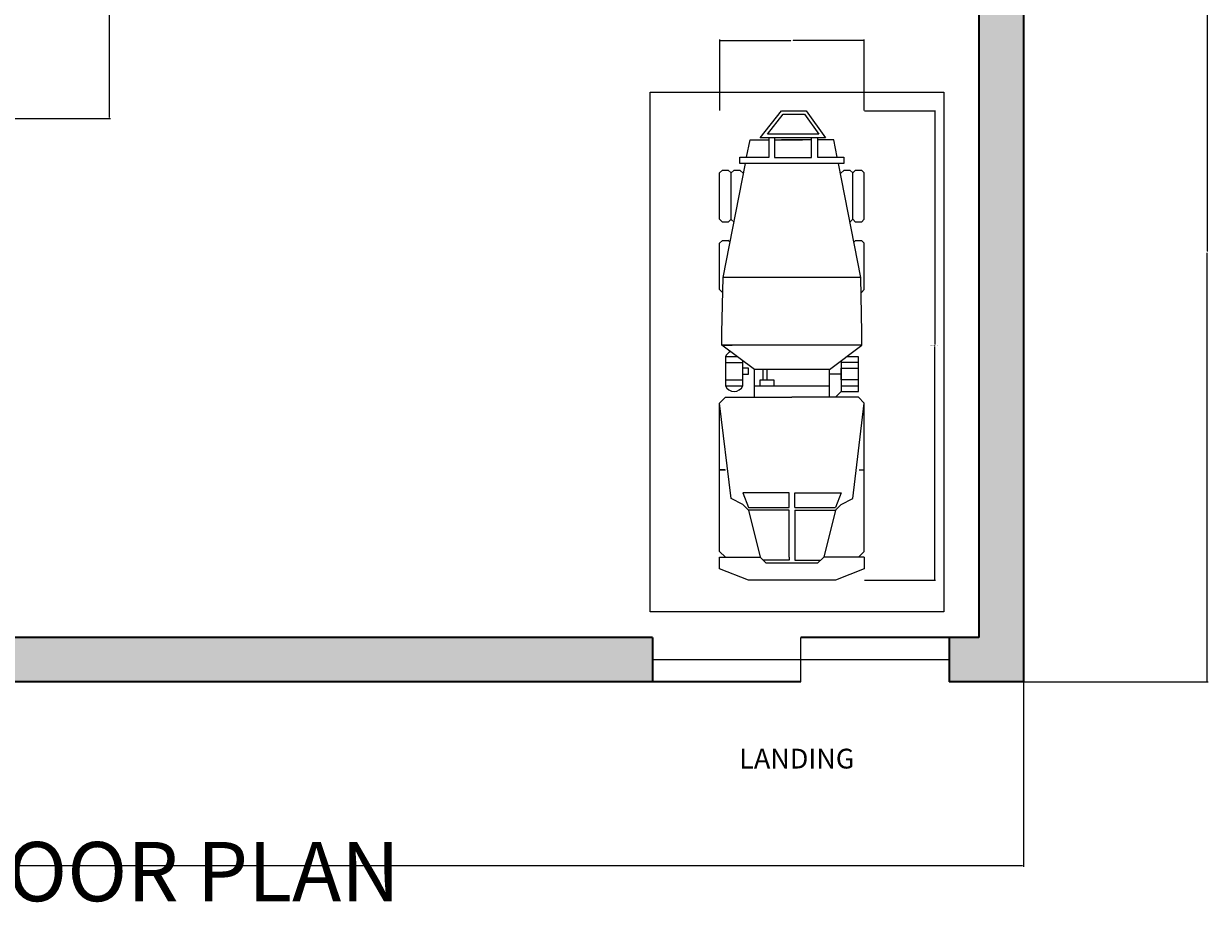
# Model space of a CAD drawing. Units: inches. Extents: x 2701 to 6846, y 811 to 2447.
# Tile 3 of 20: x 2944 to 3183, y 811 to 989. Entities that reach past the tile are written whole.
import ezdxf

# ---------------------------------------------------------------- set-up
doc = ezdxf.new("R2010")
doc.units = ezdxf.units.IN
for name, color, linetype, lineweight in [('A-ANNO-DIMS', 2, 'Continuous', 18), ('A-ANNO-TEXT', 7, 'Continuous', 18), ('A-ANNO-TITL', 7, 'Continuous', 35), ('C-PKNG', 8, 'Continuous', 18), ('C-PKNG-VEHI', 8, 'Continuous', 13), ('C-PROP', 7, 'Continuous', 35), ('C-SITE-GATE', 3, 'Continuous', 25)]:
    doc.layers.add(name, color=color, linetype=linetype, lineweight=lineweight)
doc.layers.add('C-PROP-PATT', color=18, linetype='Continuous', lineweight=13, true_color=0x000000)
doc.styles.get("Standard").update_dxf_attribs({"font": 'arial.ttf'})
doc.dimstyles.get("Standard").update_dxf_attribs({"dimtxt": 0.18, "dimasz": 0.18, "dimexe": 0.18, "dimexo": 0.0625, "dimgap": 0.09, "dimtad": 0, "dimtih": 1, "dimtoh": 1, "dimdec": 4, "dimzin": 0, "dimdsep": 46, "dimtxsty": 'Standard', "dimcen": 0.09, "dimadec": 0, "dimazin": 0, "dimtfac": 1, "dimtdec": 4, "dimtofl": 0, "dimtmove": 0, "dimatfit": 3, "dimfxl": 1, "dimtolj": 1, "dimtzin": 0, "dimarcsym": 0})

# ---------------------------------------------------------------- blocks, each defined once
blk = doc.blocks.new('A$C04877BA6')
for p, q in [((0, 1920), (192, 2400)), ((192, 2400), (384, 2400)), ((384, 2400), (384, 1728)), ((384, 2304), (480, 2400)), ((480, 2400), (1835, 2400)), ((1355, 2208), (2943, 2400)), ((1835, 2400), (2943, 2400)), ((1835, 2400), (1835, 2304)), ((1835, 2315), (1835, 2400)), ((2943, 2400), (3039, 2304)), ((3497, 1824), (3903, 2361)), ((3903, 2361), (4116, 2361)), ((3906, 2361), (3906, 2191)), ((3906, 39), (3906, 2361)), ((4116, 2361), (5025, 2341)), ((4827, 2400), (4780, 2354)), ((4827, 2400), (5595, 2400)), ((5595, 2400), (5643, 2352)), ((5994, 2400), (5946, 2352)), ((5994, 2400), (6762, 2400)), ((6762, 2400), (6810, 2352)), ((1259, 2016), (1355, 2208)), ((3039, 2304), (3039, 1200)), ((3231, 2304), (3231, 2016)), ((3711, 2304), (3231, 2304)), ((3327, 2304), (3327, 2016)), ((3615, 2304), (3615, 2016)), ((3711, 2107), (3711, 2304)), ((5025, 2341), (6922, 1972)), ((5025, 59), (5025, 2341)), ((5613, 2227), (5643, 2256)), ((5643, 2352), (5643, 2256)), ((5992, 2209), (5944, 2161)), ((5946, 2304), (5946, 2352)), ((5946, 2256), (5946, 2304)), ((5994, 2208), (5946, 2256)), ((5994, 2208), (6762, 2208)), ((6035, 2208), (6762, 2208)), ((6762, 2208), (6810, 2256)), ((6762, 2208), (6810, 2160)), ((6810, 2352), (6810, 2256)), ((1163, 1920), (1259, 2016)), ((1451, 2016), (1211, 1920)), ((1451, 1248), (1451, 2016)), ((3231, 2016), (3615, 2016)), ((3423, 2016), (3423, 1920)), ((3519, 1920), (3519, 2016)), ((3615, 2016), (3642, 2016)), ((6751, 2005), (6810, 2064)), ((6810, 2160), (6810, 2064)), ((6922, 2063), (7022, 2063)), ((6922, 340), (6922, 2063)), ((7022, 2063), (7022, 1579)), ((0, 480), (0, 1920)), ((1163, 1920), (384, 1728)), ((1163, 1248), (1163, 1920)), ((1211, 1920), (1211, 1248)), ((3039, 1824), (3497, 1824)), ((3231, 1824), (3231, 576)), ((3423, 1920), (3519, 1920)), ((3497, 1529), (3497, 1821)), ((7022, 1953), (7310, 1896)), ((7310, 1896), (7310, 1579)), ((384, 1728), (288, 1632)), ((288, 1632), (288, 768)), ((336, 1248), (336, 1680)), ((3231, 1728), (3327, 1728)), ((3327, 1728), (3327, 1624)), ((3327, 1680), (3497, 1680)), ((3327, 1624), (3327, 1500)), ((3493, 1617), (3332, 1617)), ((7022, 1579), (7348, 1579)), ((7348, 1726), (7795, 1373)), ((7348, 642), (7348, 1726)), ((7406, 755), (7406, 1607)), ((7406, 1607), (7737, 1345)), ((3327, 1500), (3231, 1500)), ((3497, 576), (3497, 1529)), ((7018, 1491), (7018, 877)), ((7348, 1491), (7018, 1491)), ((7310, 1491), (7310, 1026)), ((384, 1248), (336, 1248)), ((384, 1248), (1163, 1248)), ((1211, 1248), (1451, 1248)), ((3039, 96), (3039, 1200)), ((7310, 877), (7310, 1374)), ((7737, 1345), (7737, 993)), ((7795, 1373), (7795, 963)), ((384, 1152), (336, 1152)), ((336, 1152), (336, 720)), ((1163, 1152), (384, 1152)), ((1163, 1152), (1163, 480)), ((1211, 1152), (1211, 480)), ((1211, 1152), (1451, 1152)), ((1451, 1152), (1451, 384)), ((7737, 993), (7406, 755)), ((7018, 877), (7348, 877)), ((7795, 963), (7348, 642)), ((384, 672), (288, 768)), ((384, 0), (384, 672)), ((1163, 480), (384, 672)), ((7022, 774), (7022, 340)), ((7348, 774), (7022, 774)), ((7310, 504), (7310, 774)), ((192, 0), (0, 480)), ((1163, 480), (1259, 384)), ((1451, 384), (1211, 480)), ((3039, 576), (3497, 576)), ((3039, 480), (3135, 384)), ((3423, 384), (3423, 576)), ((3497, 576), (3903, 39)), ((5025, 59), (6922, 428)), ((6751, 395), (6810, 336)), ((7022, 447), (7310, 504)), ((1259, 384), (1355, 192)), ((3135, 384), (3135, 192)), ((3642, 384), (3135, 384)), ((3231, 384), (3231, 192)), ((3327, 96), (3327, 384)), ((3327, 384), (3519, 384)), ((3519, 384), (3519, 96)), ((3615, 96), (3615, 384)), ((3711, 96), (3711, 293)), ((5994, 192), (5948, 238)), ((6762, 192), (6810, 240)), ((6810, 336), (6810, 240)), ((7022, 340), (6922, 340)), ((384, 96), (480, 0)), ((1355, 192), (2943, 0)), ((1835, 85), (1835, 0)), ((2943, 0), (3039, 96)), ((3135, 192), (3135, 96)), ((3135, 96), (3711, 96)), ((3231, 192), (3231, 96)), ((3231, 96), (3327, 96)), ((3519, 96), (3615, 96)), ((3903, 39), (4116, 39)), ((4116, 39), (5025, 59)), ((4827, 0), (4780, 46)), ((5595, 0), (5643, 48)), ((5613, 173), (5643, 144)), ((5643, 144), (5643, 48)), ((5946, 144), (5994, 192)), ((5946, 96), (5946, 144)), ((5946, 48), (5946, 96)), ((5994, 0), (5946, 48)), ((5994, 192), (6762, 192)), ((6035, 192), (6762, 192)), ((6762, 192), (6810, 144)), ((6762, 0), (6810, 48)), ((6810, 144), (6810, 48)), ((384, 0), (192, 0)), ((480, 0), (1835, 0)), ((1835, 0), (2943, 0)), ((4827, 0), (5595, 0)), ((5994, 0), (6762, 0))]:
    blk.add_line(p, q)
for centre, radius, start, end in [((3291, 2160), 156, 112.6199, 247.3801), ((3655, 2163), 152, 21.8638, 68.3852), ((3655, 2163), 152, 254.7449, 263.8588)]:
    blk.add_arc(centre, radius, start, end)
blk = doc.blocks.new('*D63')
at = {"layer": 'A-ANNO-DIMS', "color": 0, "lineweight": -2, "transparency": 16777216}
for p, q in [((3113.86, 971.61), (3128.23, 971.61)), ((3128.05, 971.43), (3128.05, 924.3)), ((3128.05, 876.8), (3128.05, 923.93)), ((3113.86, 876.62), (3128.23, 876.62))]:
    blk.add_line(p, q, dxfattribs=at)
at = {"layer": 'A-ANNO-DIMS', "color": 0, "transparency": 16777216}
for points in [[(3128.02, 971.43), (3128.08, 971.43), (3128.05, 971.61)], [(3128.02, 876.8), (3128.08, 876.8), (3128.05, 876.62)]]:
    blk.add_solid(points, dxfattribs=at)
at = {"layer": 'Defpoints', "color": 0, "transparency": 16777216}
for p in [(3113.8, 971.61), (3128.05, 971.61), (3113.8, 876.62)]:
    blk.add_point(p, dxfattribs=at)
at = {"layer": 'A-ANNO-DIMS', "color": 0, "transparency": 16777216, "insert": (3128.05, 924.12), "char_height": 0.18, "attachment_point": 5}
blk.add_mtext('\\A1;TWO-WHEELER 95', dxfattribs=at)
blk = doc.blocks.new('*D64')
at = {"layer": 'A-ANNO-DIMS', "color": 0, "lineweight": -2, "transparency": 16777216}
for p, q in [((3084.56, 971.68), (3084.56, 986.04)), ((3084.74, 985.86), (3098.96, 985.86)), ((3113.62, 985.86), (3099.4, 985.86)), ((3113.8, 971.68), (3113.8, 986.04))]:
    blk.add_line(p, q, dxfattribs=at)
at = {"layer": 'A-ANNO-DIMS', "color": 0, "transparency": 16777216}
for points in [[(3084.74, 985.89), (3084.74, 985.83), (3084.56, 985.86)], [(3113.62, 985.89), (3113.62, 985.83), (3113.8, 985.86)]]:
    blk.add_solid(points, dxfattribs=at)
at = {"layer": 'Defpoints', "color": 0, "transparency": 16777216}
for p in [(3084.56, 985.86), (3084.56, 971.61), (3113.8, 971.61)]:
    blk.add_point(p, dxfattribs=at)
at = {"layer": 'A-ANNO-DIMS', "color": 0, "transparency": 16777216, "insert": (3099.18, 985.86), "char_height": 0.18, "attachment_point": 5}
blk.add_mtext('\\A1;29', dxfattribs=at)
blk = doc.blocks.new('*D65')
at = {"layer": 'A-ANNO-DIMS', "color": 0, "lineweight": -2, "transparency": 16777216}
for p, q in [((2737.97, 855.99), (2737.97, 818.67)), ((3145.97, 855.99), (3145.97, 818.67)), ((2738.15, 818.85), (2941.68, 818.85)), ((3145.79, 818.85), (2942.26, 818.85))]:
    blk.add_line(p, q, dxfattribs=at)
at = {"layer": 'A-ANNO-DIMS', "color": 0, "transparency": 16777216}
for points in [[(2738.15, 818.88), (2738.15, 818.82), (2737.97, 818.85)], [(3145.79, 818.88), (3145.79, 818.82), (3145.97, 818.85)]]:
    blk.add_solid(points, dxfattribs=at)
at = {"layer": 'Defpoints', "color": 0, "transparency": 16777216}
for p in [(2737.97, 856.05), (3145.97, 856.05), (3145.97, 818.85)]:
    blk.add_point(p, dxfattribs=at)
at = {"layer": 'A-ANNO-DIMS', "color": 0, "transparency": 16777216, "insert": (2941.97, 818.85), "char_height": 0.18, "attachment_point": 5}
blk.add_mtext('\\A1;408', dxfattribs=at)
blk = doc.blocks.new('*D70')
at = {"layer": 'A-ANNO-DIMS', "color": 0, "lineweight": -2, "transparency": 16777216}
for p, q in [((3092.03, 1030.05), (3183.35, 1030.05)), ((3183.17, 1029.87), (3183.17, 943.23)), ((3183.17, 856.23), (3183.17, 942.87)), ((3146.03, 856.05), (3183.35, 856.05))]:
    blk.add_line(p, q, dxfattribs=at)
at = {"layer": 'A-ANNO-DIMS', "color": 0, "transparency": 16777216}
for points in [[(3183.14, 1029.87), (3183.2, 1029.87), (3183.17, 1030.05)], [(3183.14, 856.23), (3183.2, 856.23), (3183.17, 856.05)]]:
    blk.add_solid(points, dxfattribs=at)
at = {"layer": 'Defpoints', "color": 0, "transparency": 16777216}
for p in [(3091.97, 1030.05), (3183.17, 1030.05), (3145.97, 856.05)]:
    blk.add_point(p, dxfattribs=at)
at = {"layer": 'A-ANNO-DIMS', "color": 0, "transparency": 16777216, "insert": (3183.17, 943.05), "char_height": 0.18, "attachment_point": 5}
blk.add_mtext('\\A1;174', dxfattribs=at)
blk = doc.blocks.new('*D79')
at = {"layer": 'A-ANNO-DIMS', "color": 0, "lineweight": -2, "transparency": 16777216}
for p, q in [((2924.03, 1030.05), (2961.35, 1030.05)), ((2961.17, 1029.87), (2961.17, 1000.23)), ((2961.17, 970.23), (2961.17, 999.87)), ((2924.03, 970.05), (2961.35, 970.05))]:
    blk.add_line(p, q, dxfattribs=at)
at = {"layer": 'A-ANNO-DIMS', "color": 0, "transparency": 16777216}
for points in [[(2961.14, 1029.87), (2961.2, 1029.87), (2961.17, 1030.05)], [(2961.14, 970.23), (2961.2, 970.23), (2961.17, 970.05)]]:
    blk.add_solid(points, dxfattribs=at)
at = {"layer": 'Defpoints', "color": 0, "transparency": 16777216}
for p in [(2923.97, 1030.05), (2923.97, 970.05), (2961.17, 970.05)]:
    blk.add_point(p, dxfattribs=at)
at = {"layer": 'A-ANNO-DIMS', "color": 0, "transparency": 16777216, "insert": (2961.17, 1000.05), "char_height": 0.18, "attachment_point": 5}
blk.add_mtext('\\A1;60', dxfattribs=at)

msp = doc.modelspace()

# ---------------------------------------------------------------- hatches: boundary and pattern name
at = {"layer": 'C-PROP-PATT'}
h = msp.add_hatch(color=256, dxfattribs=at)
h.dxf.hatch_style = 1
h.paths.add_polyline_path([(3145.97, 1504.05), (2737.97, 1504.05), (2737.97, 967.05), (2746.97, 967.05), (2746.97, 1495.05), (3136.97, 1495.05), (3136.97, 865.05), (3130.97, 865.05), (3130.97, 856.05), (3145.97, 856.05)])
h.paths.add_polyline_path([(3070.97, 865.05), (2746.97, 865.05), (2746.97, 871.05), (2737.97, 871.05), (2737.97, 856.05), (3070.97, 856.05)], flags=17)

# ---------------------------------------------------------------- linework, layer by layer
at = {"layer": 'C-PKNG'}
msp.add_lwpolyline([(3070.48, 975.36), (3129.9, 975.36), (3129.9, 870.21), (3070.48, 870.21)], close=True, dxfattribs=at)
at = {"layer": 'C-PROP'}
for p, q in [((3145.97, 1504.05), (3145.97, 856.05)), ((3136.97, 1495.05), (3136.97, 865.05)), ((3070.97, 865.05), (2746.97, 865.05)), ((3070.97, 865.05), (3070.97, 856.05)), ((3136.97, 865.05), (3100.97, 865.05)), ((3130.97, 865.05), (3130.97, 856.05)), ((3100.97, 856.05), (2737.97, 856.05)), ((3145.97, 856.05), (3130.97, 856.05))]:
    msp.add_line(p, q, dxfattribs=at)
at = {"layer": 'C-SITE-GATE'}
for p, q in [((3100.97, 856.05), (3100.97, 865.05)), ((3130.97, 860.55), (3070.97, 860.55))]:
    msp.add_line(p, q, dxfattribs=at)

# ---------------------------------------------------------------- block references
at = {"layer": 'C-PKNG-VEHI', "xscale": 0.012186258168831, "yscale": 0.012186258168831, "zscale": 0.012186258168831, "rotation": 90}
msp.add_blockref('A$C04877BA6', (3113.8, 876.62), dxfattribs=at)

# ---------------------------------------------------------------- texts
at = {"layer": 'A-ANNO-TEXT', "insert": (3088.52, 842.54), "char_height": 4, "attachment_point": 1}
msp.add_mtext_dynamic_manual_height_columns('{\\fTimes New Roman|b0|i0|c0|p18;LANDING}', width=25.9311, gutter_width=12.5, heights=[0], dxfattribs=at)
at = {"layer": 'A-ANNO-TITL', "insert": (2850.15, 823.68), "char_height": 12, "attachment_point": 1}
msp.add_mtext_dynamic_manual_height_columns('{\\fTimes New Roman|b0|i0|c0|p18;GROUND FLOOR PLAN}', width=192.9852, gutter_width=12.5, heights=[0], dxfattribs=at)

# ---------------------------------------------------------------- dimensions: what is measured, and where the dimension line sits
at = {"layer": 'A-ANNO-DIMS'}
for base, p1, p2, angle, picture, middle in [((2961.17, 970.05), (2923.97, 1030.05), (2923.97, 970.05), 270, '*D79', (2961.17, 1000.05)), ((3183.17, 1030.05), (3145.97, 856.05), (3091.97, 1030.05), 90, '*D70', (3183.17, 943.05)), ((3084.56, 985.86), (3113.8, 971.61), (3084.56, 971.61), 180, '*D64', (3099.18, 985.86))]:
    dim = msp.add_linear_dim(base=base, p1=p1, p2=p2, angle=angle, dimstyle='Standard', override={"dimdec": 0, "dimlfac": 1, "dimrnd": 0, "dimzin": 0, "dimdsep": 46, "dimlunit": 2}, dxfattribs=at)
    dim.commit()
    dim.dimension.update_dxf_attribs({"geometry": picture, "text_midpoint": middle})
dim = msp.add_linear_dim(base=(3128.05, 971.61), p1=(3113.8, 876.62), p2=(3113.8, 971.61), angle=90, text='TWO-WHEELER <>', dimstyle='Standard', override={"dimdec": 0, "dimlfac": 1, "dimrnd": 0, "dimzin": 0, "dimdsep": 46, "dimlunit": 2}, dxfattribs=at)
dim.commit()
dim.dimension.update_dxf_attribs({"geometry": '*D63', "text_midpoint": (3128.05, 924.12)})
dim = msp.add_linear_dim(base=(3145.97, 818.85), p1=(2737.97, 856.05), p2=(3145.97, 856.05), dimstyle='Standard', override={"dimdec": 0, "dimlfac": 1, "dimrnd": 0, "dimzin": 0, "dimdsep": 46, "dimlunit": 2}, dxfattribs=at)
dim.commit()
dim.dimension.update_dxf_attribs({"geometry": '*D65', "text_midpoint": (2941.97, 818.85)})

doc.saveas('drawing.dxf')
